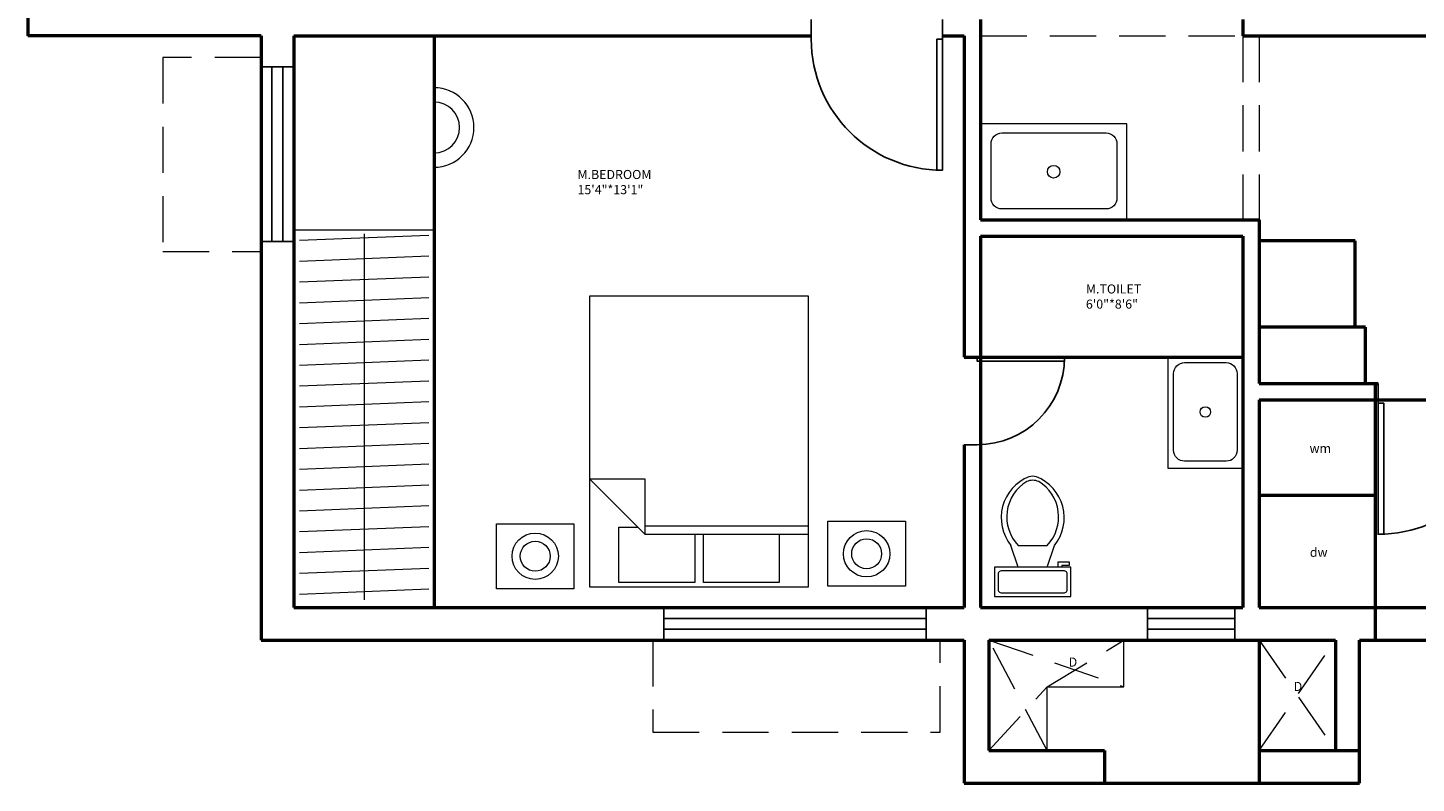
# Model space of a CAD drawing. Units: inches. Extents: x 4795 to 6024, y 2716 to 5025.
# Tile 12 of 19: x 4795 to 5177, y 4469 to 4676. Entities that reach past the tile are written whole.
import ezdxf

# ---------------------------------------------------------------- set-up
doc = ezdxf.new("R2010")
doc.units = ezdxf.units.IN
doc.linetypes.add('DASHED', pattern=[19.05, 12.7, -6.35])
for name, color, linetype, lineweight in [('A-ANNO-TEXT', 7, 'Continuous', 18), ('A-AREA-IDEN', 3, 'Continuous', 18), ('A-DOOR', 4, 'Continuous', 25), ('A-FLOR-FIXT', 9, 'Continuous', 18), ('A-FURN', 8, 'Continuous', 18), ('A-GLAZ', 4, 'Continuous', 25), ('A-WALL', 7, 'Continuous', 50), ('A-WALL-OVHD', 8, 'DASHED', 18)]:
    doc.layers.add(name, color=color, linetype=linetype, lineweight=lineweight)
doc.styles.get("Standard").update_dxf_attribs({"font": 'arial.ttf'})

# ---------------------------------------------------------------- blocks, each defined once
blk = doc.blocks.new('*U2')
for p, q in [((0, 0), (0, -6)), ((40, 0), (40, -6))]:
    blk.add_line(p, q)
blk.add_lwpolyline([(0, 0), (0, 40), (1.75, 40), (1.75, 0)], close=True)
blk.add_arc((0, 0), 40, 0, 90)
blk = doc.blocks.new('Bed - Queen')
for p, q in [((0, -80.00003), (0, 0)), ((0, 0), (59.99999, 0)), ((59.99999, 0), (59.99999, -80.00003)), ((7.99999, -1.2), (28.79998, -1.2)), ((7.99999, -14.4), (7.99999, -1.2)), ((28.79998, -1.2), (28.79998, -14.4)), ((31.19999, -1.2), (51.99999, -1.2)), ((31.19999, -14.4), (31.19999, -1.2)), ((51.99999, -1.2), (51.99999, -16.4)), ((0, -14.4), (44.8, -14.4)), ((59.99999, -29.6), (44.8, -14.4)), ((44.8, -14.4), (44.8, -29.6)), ((44.8, -16.8), (0, -16.8)), ((51.99999, -16.4), (46.79936, -16.4)), ((44.8, -29.6), (59.99999, -29.6)), ((59.99999, -80.00003), (0, -80.00003))]:
    blk.add_line(p, q)
blk = doc.blocks.new('Toilet - top')
for p, q in [((9.5, -6), (9.5, -2)), ((-10, -8.5), (-8, -8.5)), ((-10, -9.5), (-10, -8.5)), ((-7, -9.5), (-10, -9.5)), ((-8, -8.5), (-8, -8)), ((-7, -8), (-7, -9.5)), ((-4, -8), (-6, -14)), ((4, -8), (6, -14)), ((4, -14), (-4, -14))]:
    blk.add_line(p, q)
blk.add_lwpolyline([(10.5, -8), (10.5, 0), (-10.5, 0), (-10.5, -8)], close=True)
for points in [[(-9.5, -2), (-9.5, -6)], [(8.5, -1), (-8.5, -1)], [(-8.5, -7), (8.5, -7)]]:
    blk.add_lwpolyline(points)
for centre, radius, start, end in [((-8.62, -1.88), 0.884, 81.8699, 188.1301), ((8.62, -1.88), 0.884, 351.8699, 98.1301), ((-8.62, -6.12), 0.884, 171.8699, 278.1301), ((8.62, -6.12), 0.884, 261.8699, 8.1301), ((3.52, -21.58), 12.17, 141.4691, 247.9714), ((4.2, -21.82), 11.33, 136.3677, 238.9468), ((-3.52, -21.58), 12.17, 292.0284, 38.5307), ((-4.2, -21.82), 11.33, 301.053, 43.6321), ((0, -27.88), 4, 245.7318, 294.2682), ((0, -29), 4, 254.8605, 285.1395)]:
    blk.add_arc(centre, radius, start, end)
blk = doc.blocks.new('WIN-48')
for p, q in [((0, 0), (0, 48)), ((0, 48), (9, 48)), ((3, 0), (3, 48)), ((6, 48), (6, 0)), ((9, 48), (9, 0)), ((9, 0), (0, 0))]:
    blk.add_line(p, q)
blk = doc.blocks.new('WIN-72')
for p, q in [((0, 0), (0, 9)), ((0, 9), (72, 9)), ((72, 9), (72, 0)), ((0, 6), (72, 6)), ((72, 3), (0, 3)), ((72, 0), (0, 0))]:
    blk.add_line(p, q)
blk = doc.blocks.new('WIN-24')
for p, q in [((0, 0), (0, 9)), ((0, 9), (24, 9)), ((24, 9), (24, 0)), ((0, 6), (24, 6)), ((24, 3), (0, 3)), ((24, 0), (0, 0))]:
    blk.add_line(p, q)

msp = doc.modelspace()

# ---------------------------------------------------------------- linework, layer by layer
at = {"layer": 'A-FLOR-FIXT'}
for points in [[(5056.97, 4623.48), (5097.17, 4623.48), (5097.17, 4649.88), (5056.97, 4649.88)], [(5128.97, 4585.7), (5108.42, 4585.7), (5108.42, 4555.23), (5128.97, 4555.23)]]:
    msp.add_lwpolyline(points, close=True, dxfattribs=at)
for points in [[(5062.88, 4647.33), (5091.45, 4647.33, -0.414214), (5094.45, 4644.33), (5094.45, 4629.46, -0.414214), (5091.45, 4626.46), (5062.88, 4626.46, -0.414214), (5059.88, 4629.46), (5059.88, 4644.33, -0.414214)], [(5113, 4584.23), (5124.45, 4584.23, -0.414214), (5127.45, 4581.23), (5127.45, 4560.16, -0.414214), (5124.45, 4557.16), (5113, 4557.16, -0.414214), (5110, 4560.16), (5110, 4581.23, -0.414214)]]:
    msp.add_lwpolyline(points, format="xyb", close=True, dxfattribs=at)
for centre, radius in [((5077.07, 4636.68), 1.73), ((5118.72, 4570.69), 1.45)]:
    msp.add_circle(centre, radius, dxfattribs=at)
at = {"layer": 'A-FURN'}
for p, q in [((4868.47, 4620.7), (4906.98, 4620.7)), ((4870.06, 4617.85), (4905.5, 4619.28)), ((4887.78, 4619.66), (4887.78, 4519.03)), ((4870.06, 4612.13), (4905.5, 4613.57)), ((4870.06, 4606.41), (4905.5, 4607.85)), ((4870.06, 4600.7), (4905.5, 4602.13)), ((4870.06, 4594.98), (4905.5, 4596.42)), ((4870.06, 4589.26), (4905.5, 4590.7)), ((4870.06, 4583.55), (4905.5, 4584.98)), ((4870.06, 4577.83), (4905.5, 4579.27)), ((4870.06, 4572.11), (4905.5, 4573.55)), ((4870.06, 4566.4), (4905.5, 4567.83)), ((4870.06, 4560.68), (4905.5, 4562.12)), ((4870.06, 4554.96), (4905.5, 4556.4)), ((4870.06, 4549.24), (4905.5, 4550.68)), ((4870.06, 4543.53), (4905.5, 4544.96)), ((4870.06, 4537.81), (4905.5, 4539.25)), ((4870.06, 4532.09), (4905.5, 4533.53)), ((4870.06, 4526.38), (4905.5, 4527.81)), ((4870.06, 4520.66), (4905.5, 4522.1)), ((5096.38, 4495.19), (5096.38, 4507.98)), ((5075.3, 4477.69), (5075.3, 4495.19)), ((5075.3, 4495.19), (5096.38, 4495.19))]:
    msp.add_line(p, q, dxfattribs=at)
for points in [[(4924.11, 4539.97), (4945.37, 4539.97), (4945.37, 4522.14), (4924.11, 4522.14)], [(5015.1, 4540.65), (5036.37, 4540.65), (5036.37, 4522.81), (5015.1, 4522.81)]]:
    msp.add_lwpolyline(points, close=True, dxfattribs=at)
for centre, radius in [((4934.74, 4531.05), 6.37), ((5025.73, 4531.73), 6.37), ((4934.74, 4531.05), 4.11), ((5025.73, 4531.73), 4.11)]:
    msp.add_circle(centre, radius, dxfattribs=at)
for radius in [10.92, 6.99]:
    msp.add_arc((4906.98, 4648.82), radius, 270, 90, dxfattribs=at)
at = {"layer": 'A-WALL'}
for p, q in [((4795.42, 4820.98), (4795.42, 4673.98)), ((5056.97, 4678.48), (5056.97, 4623.48)), ((5128.97, 4678.48), (5128.97, 4673.98)), ((4859.47, 4673.98), (4795.42, 4673.98)), ((4859.47, 4673.98), (4859.47, 4507.98)), ((4868.47, 4673.98), (5010.54, 4673.98)), ((4868.47, 4673.98), (4868.47, 4516.98)), ((4906.98, 4673.98), (4906.98, 4516.98)), ((5046.54, 4673.98), (5052.47, 4673.98)), ((5052.47, 4673.98), (5052.47, 4585.7)), ((5128.97, 4673.98), (5277.97, 4673.98)), ((5056.97, 4623.48), (5133.47, 4623.48)), ((5133.47, 4623.48), (5133.47, 4578.48)), ((5056.97, 4618.98), (5128.97, 4618.98)), ((5056.97, 4618.98), (5056.97, 4516.98)), ((5128.97, 4618.98), (5128.97, 4516.98)), ((5159.88, 4617.73), (5133.47, 4617.73)), ((5159.88, 4593.95), (5159.88, 4617.73)), ((5162.73, 4593.95), (5133.47, 4593.95)), ((5162.73, 4578.48), (5162.73, 4593.95)), ((5052.47, 4585.7), (5128.97, 4585.7)), ((5133.47, 4578.48), (5166.12, 4578.48)), ((5165.35, 4578.48), (5165.35, 4516.98)), ((5133.47, 4573.98), (5277.97, 4573.98)), ((5133.47, 4573.98), (5133.47, 4516.98)), ((5052.47, 4561.7), (5052.47, 4516.98)), ((5165.35, 4547.73), (5133.47, 4547.73)), ((4868.47, 4516.98), (5052.47, 4516.98)), ((5056.97, 4516.98), (5128.97, 4516.98)), ((5133.47, 4516.98), (5277.97, 4516.98)), ((5165.35, 4516.98), (5165.35, 4507.98)), ((4859.47, 4507.98), (5052.47, 4507.98)), ((5052.47, 4507.98), (5052.47, 4468.69)), ((5059.32, 4507.98), (5059.32, 4477.69)), ((5059.32, 4507.98), (5154.41, 4507.98)), ((5133.47, 4507.98), (5133.47, 4468.69)), ((5154.41, 4507.98), (5154.41, 4477.69)), ((5161.01, 4468.69), (5161.01, 4507.98)), ((5161.01, 4507.98), (5286.97, 4507.98)), ((5059.32, 4477.69), (5090.99, 4477.69)), ((5090.99, 4477.69), (5090.99, 4468.69)), ((5133.47, 4477.69), (5161.01, 4477.69)), ((5052.47, 4468.69), (5161.01, 4468.69))]:
    msp.add_line(p, q, dxfattribs=at)
at = {"layer": 'A-WALL-OVHD'}
for p, q in [((5056.97, 4673.98), (5128.97, 4673.98)), ((5128.97, 4673.98), (5128.97, 4623.48)), ((5133.47, 4673.98), (5133.47, 4623.48)), ((4859.47, 4668.1), (4832.53, 4668.1)), ((4832.53, 4668.1), (4832.53, 4614.78)), ((4832.53, 4614.78), (4859.47, 4614.78)), ((4967.07, 4507.98), (4967.07, 4482.69)), ((5045.91, 4482.69), (5045.91, 4507.98)), ((5075.3, 4477.69), (5059.32, 4507.98)), ((5059.32, 4507.98), (5096.38, 4495.19)), ((5075.3, 4495.19), (5096.38, 4507.98)), ((5133.47, 4507.98), (5154.41, 4477.69)), ((5133.47, 4477.69), (5154.41, 4507.98)), ((5059.32, 4477.69), (5075.3, 4495.19)), ((4967.07, 4482.69), (5045.91, 4482.69))]:
    msp.add_line(p, q, dxfattribs=at)

# ---------------------------------------------------------------- block references
at = {"layer": 'A-DOOR'}
for p, xscale, yscale, zscale, rotation in [((5046.54, 4673.08), 0.9, 0.9, 0.9, 180), ((5056.07, 4585.7), 0.6, 0.6, 0.6, 270), ((5166.12, 4573.08), -0.9, 0.9, 0.9, 180)]:
    msp.add_blockref('*U2', p, dxfattribs=dict(at, xscale=xscale, yscale=yscale, zscale=zscale, rotation=rotation))
at = {"layer": 'A-FLOR-FIXT', "rotation": 180}
msp.add_blockref('Toilet - top', (5071.32, 4520.03), dxfattribs=at)
at = {"layer": 'A-FURN', "rotation": 180}
msp.add_blockref('Bed - Queen', (5009.72, 4522.6), dxfattribs=at)
at = {"layer": 'A-GLAZ'}
msp.add_blockref('WIN-48', (4859.47, 4617.53), dxfattribs=at)
at = {"layer": 'A-GLAZ', "rotation": 180}
for name, p in [('WIN-72', (5042.09, 4516.98)), ('WIN-24', (5126.8, 4516.98))]:
    msp.add_blockref(name, p, dxfattribs=at)

# ---------------------------------------------------------------- texts
at = {"layer": 'A-ANNO-TEXT', "char_height": 2.5, "attachment_point": 1}
for s, width, insert in [('wm', 14.5674, (5147.33, 4561.95)), ('dw', 14.0253, (5147.41, 4533.39)), ('D', 2.8218, (5081.2, 4503.22)), ('D', 1.6038, (5142.97, 4496.53))]:
    msp.add_mtext_dynamic_manual_height_columns(s, width=width, gutter_width=12.5, heights=[0], dxfattribs=dict(at, insert=insert))
at = {"layer": 'A-AREA-IDEN', "char_height": 2.5, "attachment_point": 1}
for s, width, insert in [('M.BEDROOM\\P15\'4"*13\'1"', 71.106, (4946.34, 4637.17)), ('M.TOILET\\P6\'0"*8\'6"', 46.3595, (5085.93, 4605.73))]:
    msp.add_mtext_dynamic_manual_height_columns(s, width=width, gutter_width=12.5, heights=[0], dxfattribs=dict(at, insert=insert))

doc.saveas('drawing.dxf')
